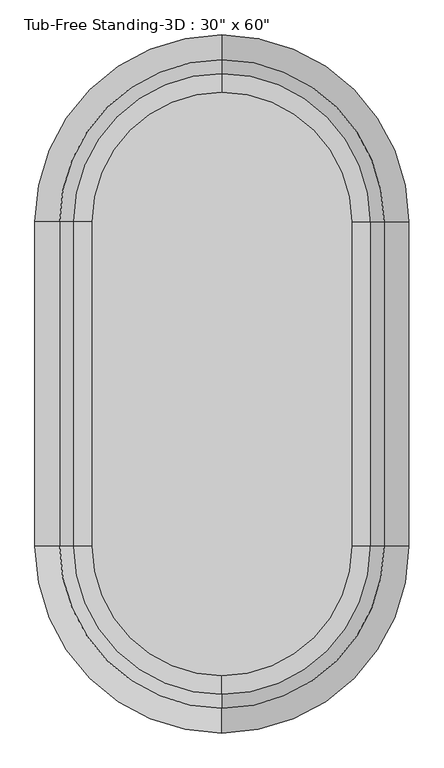
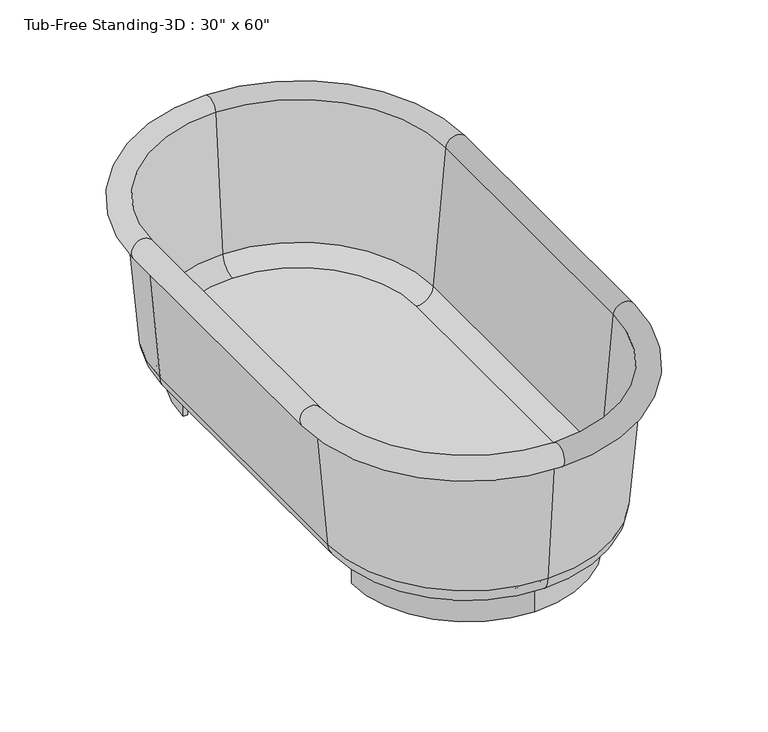
"""IFC4 building model written with IfcOpenShell, lengths in millimetres: flow terminal geometry."""

from ifc_helpers import new_model, si_unit, point, frame, frame_2d, origin, origin_with_axes, place, context, project, spatial, polyline, circle_curve, ellipse_curve, trimmed, segment, composite_curve, outline, extrude, source, transform, mapped, element, save
from ifc_brep_helpers import plane_surface, cylinder_surface, revolved_surface, advanced_brep


def flow_terminal_a2f06f5b(model_context):
    return source(origin(), model_context, "Body", "SolidModel", [
        extrude(outline(composite_curve([segment(trimmed(circle_curve(frame_2d((0.0, 330.2)), 254.0), [point((0.0, 584.2))], [point((-254.0, 330.2))], True, "CARTESIAN"), True, "CONTINUOUS"), segment(polyline([(-254.0, 330.2), (-264.2824236, 330.2)]), True, "CONTINUOUS"), segment(trimmed(circle_curve(frame_2d((0.0, 330.2)), 264.2824236), [point((-264.2824236, 330.2))], [point((0.0, 594.4824236))], False, "CARTESIAN"), True, "CONTINUOUS"), segment(trimmed(circle_curve(frame_2d((0.0, 330.2)), 264.2824236), [point((0.0, 594.4824236))], [point((264.2824236, 330.2))], False, "CARTESIAN"), True, "CONTINUOUS"), segment(polyline([(264.2824236, 330.2), (254.0, 330.2)]), True, "CONTINUOUS"), segment(trimmed(circle_curve(frame_2d((0.0, 330.2)), 254.0), [point((254.0, 330.2))], [point((0.0, 584.2))], True, "CARTESIAN"), True, "CONTINUOUS")], self_intersect=False)), origin_with_axes(), (0.0, 0.0, 1.0), 63.5),
        extrude(outline(composite_curve([segment(trimmed(circle_curve(frame_2d((0.0, -330.2)), 264.2824236), [point((0.0, -594.4824236))], [point((-264.2824236, -330.2))], False, "CARTESIAN"), True, "CONTINUOUS"), segment(polyline([(-264.2824236, -330.2), (-254.0, -330.2)]), True, "CONTINUOUS"), segment(trimmed(circle_curve(frame_2d((0.0, -330.2)), 254.0), [point((-254.0, -330.2))], [point((0.0, -584.2))], True, "CARTESIAN"), True, "CONTINUOUS"), segment(trimmed(circle_curve(frame_2d((0.0, -330.2)), 254.0), [point((0.0, -584.2))], [point((254.0, -330.2))], True, "CARTESIAN"), True, "CONTINUOUS"), segment(polyline([(254.0, -330.2), (264.2824236, -330.2)]), True, "CONTINUOUS"), segment(trimmed(circle_curve(frame_2d((0.0, -330.2)), 264.2824236), [point((264.2824236, -330.2))], [point((0.0, -594.4824236))], False, "CARTESIAN"), True, "CONTINUOUS")], self_intersect=False)), origin_with_axes(), (0.0, 0.0, 1.0), 63.5),
        extrude(outline(composite_curve([segment(polyline([(-264.2824236, -330.2), (-264.2824236, 330.2)]), True, "CONTINUOUS"), segment(trimmed(circle_curve(frame_2d((0.0, 330.2)), 264.2824236), [point((-264.2824236, 330.2))], [point((0.0, 594.4824236))], False, "CARTESIAN"), True, "CONTINUOUS"), segment(trimmed(circle_curve(frame_2d((0.0, 330.2)), 264.2824236), [point((0.0, 594.4824236))], [point((264.2824236, 330.2))], False, "CARTESIAN"), True, "CONTINUOUS"), segment(polyline([(264.2824236, 330.2), (264.2824236, -330.2)]), True, "CONTINUOUS"), segment(trimmed(circle_curve(frame_2d((0.0, -330.2)), 264.2824236), [point((264.2824236, -330.2))], [point((0.0, -594.4824236))], False, "CARTESIAN"), True, "CONTINUOUS"), segment(trimmed(circle_curve(frame_2d((0.0, -330.2)), 264.2824236), [point((0.0, -594.4824236))], [point((-264.2824236, -330.2))], False, "CARTESIAN"), True, "CONTINUOUS")], self_intersect=False)), frame((0.0, 0.0, 63.5), z_axis=(0.0, 0.0, 1.0), x_axis=(1.0, 0.0, 0.0)), (0.0, 0.0, 1.0), 15.08125),
        advanced_brep(
        [(0.0, -673.1, 406.4), (342.9, -330.2, 406.4), (355.6, -330.2, 406.4), (0.0, -685.8, 406.4), (0.0, -647.3045038, 111.5561295), (317.1045038, -330.2, 111.5561295), (0.0, -594.4824236, 63.1536107), (264.2824236, -330.2, 63.1536107), (0.0, -594.4824236, 78.0774627), (264.2824236, -330.2, 78.0774627), (0.0, -632.4374416, 112.8568289), (302.2374416, -330.2, 112.8568289), (0.0, -660.6561556, 435.3982063), (330.4561556, -330.2, 435.3982063), (-342.9, -330.2, 406.4), (-355.6, -330.2, 406.4), (-317.1045038, -330.2, 111.5561295), (-264.2824236, -330.2, 63.1536107), (-264.2824236, -330.2, 78.0774627), (-302.2374416, -330.2, 112.8568289), (-330.4561556, -330.2, 435.3982063), (-355.6, 330.2, 406.4), (-342.9, 330.2, 406.4), (-317.1045038, 330.2, 111.5561295), (-264.2824236, 330.2, 63.1536107), (-264.2824236, 330.2, 78.0774627), (-302.2374416, 330.2, 112.8568289), (-330.4561556, 330.2, 435.3982063), (0.0, 673.1, 406.4), (0.0, 685.8, 406.4), (0.0, 647.3045038, 111.5561295), (0.0, 594.4824236, 63.1536107), (0.0, 594.4824236, 78.0774627), (0.0, 632.4374416, 112.8568289), (0.0, 660.6561556, 435.3982063), (342.9, 330.2, 406.4), (355.6, 330.2, 406.4), (317.1045038, 330.2, 111.5561295), (264.2824236, 330.2, 63.1536107), (264.2824236, 330.2, 78.0774627), (302.2374416, 330.2, 112.8568289), (330.4561556, 330.2, 435.3982063)],
        [
            (0, 1, circle_curve(frame((0.0, -330.2, 406.4), z_axis=(0.0, 0.0, 1.0), x_axis=(1.0, 0.0, 0.0)), 342.9)),
            (1, 2),
            (2, 3, circle_curve(frame((0.0, -330.2, 406.4), z_axis=(0.0, 0.0, -1.0), x_axis=(1.0, 0.0, 0.0)), 355.6)),
            (3, 0),
            (4, 5, circle_curve(frame((0.0, -330.2, 111.5561295), z_axis=(0.0, 0.0, 1.0), x_axis=(1.0, 0.0, 0.0)), 317.1045038)),
            (5, 1),
            (0, 4),
            (6, 7, circle_curve(frame((0.0, -330.2, 63.1536107), z_axis=(0.0, 0.0, 1.0), x_axis=(1.0, 0.0, 0.0)), 264.2824236)),
            (7, 5, circle_curve(frame((264.2824236, -330.2, 116.1774627), z_axis=(0.0, -1.0, 0.0), x_axis=(1.0, 0.0, 0.0)), 53.023852)),
            (4, 6, circle_curve(frame((0.0, -594.4824236, 116.1774627), z_axis=(1.0, 0.0, 0.0), x_axis=(0.0, -1.0, 0.0)), 53.023852)),
            (8, 9, circle_curve(frame((0.0, -330.2, 78.0774627), z_axis=(0.0, 0.0, 1.0), x_axis=(1.0, 0.0, 0.0)), 264.2824236)),
            (9, 7),
            (6, 8),
            (10, 11, circle_curve(frame((0.0, -330.2, 112.8568289), z_axis=(0.0, 0.0, 1.0), x_axis=(1.0, 0.0, 0.0)), 302.2374416)),
            (11, 9, circle_curve(frame((264.2824236, -330.2, 116.1774627), z_axis=(0.0, 1.0, 0.0), x_axis=(1.0, 0.0, 0.0)), 38.1)),
            (8, 10, circle_curve(frame((0.0, -594.4824236, 116.1774627), z_axis=(-1.0, 0.0, 0.0), x_axis=(0.0, -1.0, 0.0)), 38.1)),
            (12, 13, circle_curve(frame((0.0, -330.2, 435.3982063), z_axis=(0.0, 0.0, 1.0), x_axis=(1.0, 0.0, 0.0)), 330.4561556)),
            (13, 11),
            (10, 12),
            (2, 13, circle_curve(frame((355.6, -330.2, 431.8), z_axis=(0.0, -1.0, 0.0), x_axis=(1.0, 0.0, 0.0)), 25.4)),
            (12, 3, circle_curve(frame((0.0, -685.8, 431.8), z_axis=(1.0, 0.0, 0.0), x_axis=(0.0, -1.0, 0.0)), 25.4)),
            (14, 0, circle_curve(frame((0.0, -330.2, 406.4), z_axis=(0.0, 0.0, 1.0), x_axis=(0.0, -1.0, 0.0)), 342.9)),
            (3, 15, circle_curve(frame((0.0, -330.2, 406.4), z_axis=(0.0, 0.0, -1.0), x_axis=(0.0, -1.0, 0.0)), 355.6)),
            (15, 14),
            (16, 4, circle_curve(frame((0.0, -330.2, 111.5561295), z_axis=(0.0, 0.0, 1.0), x_axis=(0.0, -1.0, 0.0)), 317.1045038)),
            (14, 16),
            (17, 6, circle_curve(frame((0.0, -330.2, 63.1536107), z_axis=(0.0, 0.0, 1.0), x_axis=(0.0, -1.0, 0.0)), 264.2824236)),
            (16, 17, circle_curve(frame((-264.2824236, -330.2, 116.1774627), z_axis=(0.0, -1.0, 0.0), x_axis=(-1.0, 0.0, 0.0)), 53.023852)),
            (18, 8, circle_curve(frame((0.0, -330.2, 78.0774627), z_axis=(0.0, 0.0, 1.0), x_axis=(0.0, -1.0, 0.0)), 264.2824236)),
            (17, 18),
            (19, 10, circle_curve(frame((0.0, -330.2, 112.8568289), z_axis=(0.0, 0.0, 1.0), x_axis=(0.0, -1.0, 0.0)), 302.2374416)),
            (18, 19, circle_curve(frame((-264.2824236, -330.2, 116.1774627), z_axis=(0.0, 1.0, 0.0), x_axis=(-1.0, 0.0, 0.0)), 38.1)),
            (20, 12, circle_curve(frame((0.0, -330.2, 435.3982063), z_axis=(0.0, 0.0, 1.0), x_axis=(0.0, -1.0, 0.0)), 330.4561556)),
            (19, 20),
            (20, 15, circle_curve(frame((-355.6, -330.2, 431.8), z_axis=(0.0, -1.0, 0.0), x_axis=(-1.0, 0.0, 0.0)), 25.4)),
            (15, 21),
            (21, 22),
            (22, 14),
            (22, 23),
            (23, 16),
            (23, 24, circle_curve(frame((-264.2824236, 330.2, 116.1774627), z_axis=(0.0, -1.0, 0.0), x_axis=(-1.0, 0.0, 0.0)), 53.023852)),
            (24, 17),
            (24, 25),
            (25, 18),
            (25, 26, circle_curve(frame((-264.2824236, 330.2, 116.1774627), z_axis=(0.0, 1.0, 0.0), x_axis=(-1.0, 0.0, 0.0)), 38.1)),
            (26, 19),
            (26, 27),
            (27, 20),
            (27, 21, circle_curve(frame((-355.6, 330.2, 431.8), z_axis=(0.0, -1.0, 0.0), x_axis=(-1.0, 0.0, 0.0)), 25.4)),
            (28, 22, circle_curve(frame((0.0, 330.2, 406.4), z_axis=(0.0, 0.0, 1.0), x_axis=(-1.0, 0.0, 0.0)), 342.9)),
            (21, 29, circle_curve(frame((0.0, 330.2, 406.4), z_axis=(0.0, 0.0, -1.0), x_axis=(-1.0, 0.0, 0.0)), 355.6)),
            (29, 28),
            (30, 23, circle_curve(frame((0.0, 330.2, 111.5561295), z_axis=(0.0, 0.0, 1.0), x_axis=(-1.0, 0.0, 0.0)), 317.1045038)),
            (28, 30),
            (31, 24, circle_curve(frame((0.0, 330.2, 63.1536107), z_axis=(0.0, 0.0, 1.0), x_axis=(-1.0, 0.0, 0.0)), 264.2824236)),
            (30, 31, circle_curve(frame((0.0, 594.4824236, 116.1774627), z_axis=(-1.0, 0.0, 0.0), x_axis=(0.0, 1.0, 0.0)), 53.023852)),
            (32, 25, circle_curve(frame((0.0, 330.2, 78.0774627), z_axis=(0.0, 0.0, 1.0), x_axis=(-1.0, 0.0, 0.0)), 264.2824236)),
            (31, 32),
            (33, 26, circle_curve(frame((0.0, 330.2, 112.8568289), z_axis=(0.0, 0.0, 1.0), x_axis=(-1.0, 0.0, 0.0)), 302.2374416)),
            (32, 33, circle_curve(frame((0.0, 594.4824236, 116.1774627), z_axis=(1.0, 0.0, 0.0), x_axis=(0.0, 1.0, 0.0)), 38.1)),
            (34, 27, circle_curve(frame((0.0, 330.2, 435.3982063), z_axis=(0.0, 0.0, 1.0), x_axis=(-1.0, 0.0, 0.0)), 330.4561556)),
            (33, 34),
            (34, 29, circle_curve(frame((0.0, 685.8, 431.8), z_axis=(-1.0, 0.0, 0.0), x_axis=(0.0, 1.0, 0.0)), 25.4)),
            (35, 28, circle_curve(frame((0.0, 330.2, 406.4), z_axis=(0.0, 0.0, 1.0), x_axis=(0.0, 1.0, 0.0)), 342.9)),
            (29, 36, circle_curve(frame((0.0, 330.2, 406.4), z_axis=(0.0, 0.0, -1.0), x_axis=(0.0, 1.0, 0.0)), 355.6)),
            (36, 35),
            (37, 30, circle_curve(frame((0.0, 330.2, 111.5561295), z_axis=(0.0, 0.0, 1.0), x_axis=(0.0, 1.0, 0.0)), 317.1045038)),
            (35, 37),
            (38, 31, circle_curve(frame((0.0, 330.2, 63.1536107), z_axis=(0.0, 0.0, 1.0), x_axis=(0.0, 1.0, 0.0)), 264.2824236)),
            (37, 38, circle_curve(frame((264.2824236, 330.2, 116.1774627), z_axis=(0.0, 1.0, 0.0), x_axis=(1.0, 0.0, 0.0)), 53.023852)),
            (39, 32, circle_curve(frame((0.0, 330.2, 78.0774627), z_axis=(0.0, 0.0, 1.0), x_axis=(0.0, 1.0, 0.0)), 264.2824236)),
            (38, 39),
            (40, 33, circle_curve(frame((0.0, 330.2, 112.8568289), z_axis=(0.0, 0.0, 1.0), x_axis=(0.0, 1.0, 0.0)), 302.2374416)),
            (39, 40, circle_curve(frame((264.2824236, 330.2, 116.1774627), z_axis=(0.0, -1.0, 0.0), x_axis=(1.0, 0.0, 0.0)), 38.1)),
            (41, 34, circle_curve(frame((0.0, 330.2, 435.3982063), z_axis=(0.0, 0.0, 1.0), x_axis=(0.0, 1.0, 0.0)), 330.4561556)),
            (40, 41),
            (41, 36, circle_curve(frame((355.6, 330.2, 431.8), z_axis=(0.0, 1.0, 0.0), x_axis=(1.0, 0.0, 0.0)), 25.4)),
            (36, 2),
            (1, 35),
            (5, 37),
            (7, 38),
            (9, 39),
            (11, 40),
            (13, 41),
        ],
        [
            plane_surface(frame((0.0, -330.2, 406.4), z_axis=(0.0, 0.0, -1.0), x_axis=(1.0, 0.0, 0.0))),
            revolved_surface(polyline([(342.9, -330.2, 406.4), (317.1045038, -330.2, 111.5561295)]), (0.0, -330.2, 431.8), (0.0, 0.0, -1.0)),
            revolved_surface(trimmed(ellipse_curve(frame((264.2824236, -330.2, 116.1774627), z_axis=(0.0, 1.0, 0.0), x_axis=(1.0, 0.0, 0.0)), 53.023852, 53.023852), [point((317.1045038, -330.2, 111.5561295))], [point((264.2824236, -330.2, 63.1536107))], True, "CARTESIAN"), (0.0, -330.2, 431.8), (0.0, 0.0, -1.0)),
            revolved_surface(polyline([(264.2824236, -330.2, 63.1536107), (264.2824236, -330.2, 78.07746270000001)]), (0.0, -330.2, 431.8), (0.0, 0.0, -1.0)),
            revolved_surface(trimmed(ellipse_curve(frame((264.2824236, -330.2, 116.1774627), z_axis=(0.0, -1.0, 0.0), x_axis=(1.0, 0.0, 0.0)), 38.1, 38.1), [point((264.2824236, -330.2, 78.0774627))], [point((302.2374416, -330.2, 112.8568289))], True, "CARTESIAN"), (0.0, -330.2, 431.8), (0.0, 0.0, -1.0)),
            revolved_surface(polyline([(302.2374416, -330.2, 112.8568289), (330.4561556, -330.2, 435.3982063)]), (0.0, -330.2, 431.8), (0.0, 0.0, -1.0)),
            revolved_surface(trimmed(ellipse_curve(frame((355.6, -330.2, 431.8), z_axis=(0.0, 1.0, 0.0), x_axis=(1.0, 0.0, 0.0)), 25.4, 25.4), [point((330.4561556, -330.2, 435.3982063))], [point((355.6, -330.2, 406.4))], True, "CARTESIAN"), (0.0, -330.2, 431.8), (0.0, 0.0, -1.0)),
            plane_surface(frame((0.0, -330.2, 406.4), z_axis=(0.0, 0.0, -1.0), x_axis=(0.0, -1.0, 0.0))),
            revolved_surface(polyline([(0.0, -673.1, 406.4), (0.0, -647.3045038, 111.5561295)]), (0.0, -330.2, 431.8), (0.0, 0.0, -1.0)),
            revolved_surface(trimmed(ellipse_curve(frame((0.0, -594.4824236, 116.1774627), z_axis=(1.0, 0.0, 0.0), x_axis=(0.0, -1.0, 0.0)), 53.023852, 53.023852), [point((0.0, -647.3045038, 111.5561295))], [point((0.0, -594.4824236, 63.1536107))], True, "CARTESIAN"), (0.0, -330.2, 431.8), (0.0, 0.0, -1.0)),
            revolved_surface(polyline([(0.0, -594.4824236, 63.1536107), (0.0, -594.4824236, 78.07746270000001)]), (0.0, -330.2, 431.8), (0.0, 0.0, -1.0)),
            revolved_surface(trimmed(ellipse_curve(frame((0.0, -594.4824236, 116.1774627), z_axis=(-1.0, 0.0, 0.0), x_axis=(0.0, -1.0, 0.0)), 38.1, 38.1), [point((0.0, -594.4824236, 78.0774627))], [point((0.0, -632.4374416, 112.8568289))], True, "CARTESIAN"), (0.0, -330.2, 431.8), (0.0, 0.0, -1.0)),
            revolved_surface(polyline([(0.0, -632.4374416, 112.8568289), (0.0, -660.6561556, 435.3982063)]), (0.0, -330.2, 431.8), (0.0, 0.0, -1.0)),
            revolved_surface(trimmed(ellipse_curve(frame((0.0, -685.8, 431.8), z_axis=(1.0, 0.0, 0.0), x_axis=(0.0, -1.0, 0.0)), 25.4, 25.4), [point((0.0, -660.6561556, 435.3982063))], [point((0.0, -685.8, 406.4))], True, "CARTESIAN"), (0.0, -330.2, 431.8), (0.0, 0.0, -1.0)),
            plane_surface(frame((-355.6, -330.2, 406.4), z_axis=(0.0, 0.0, -1.0), x_axis=(0.0, 1.0, 0.0))),
            plane_surface(frame((-342.9, -330.2, 406.4), z_axis=(-0.9961946980917455, 0.0, -0.08715574274765871), x_axis=(0.0, 1.0, 0.0))),
            cylinder_surface(frame((-264.2824236, -330.2, 116.1774627), z_axis=(0.0, -1.0, 0.0), x_axis=(-1.0, 0.0, 0.0)), 53.023852),
            plane_surface(frame((-264.2824236, -330.2, 63.1536107), z_axis=(1.0, 0.0, 0.0), x_axis=(0.0, 1.0, 0.0))),
            revolved_surface(polyline([(-302.38242360000004, 330.2, 116.1774627), (-302.38242360000004, -330.2, 116.1774627)]), (-264.2824236, -330.2, 116.1774627), (0.0, 1.0, 0.0)),
            plane_surface(frame((-302.2374416, -330.2, 112.8568289), z_axis=(0.9961946980917458, 0.0, 0.08715574274765651), x_axis=(0.0, 1.0, 0.0))),
            cylinder_surface(frame((-355.6, -330.2, 431.8), z_axis=(0.0, -1.0, 0.0), x_axis=(-1.0, 0.0, 0.0)), 25.4),
            plane_surface(frame((0.0, 330.2, 406.4), z_axis=(0.0, 0.0, -1.0), x_axis=(-1.0, 0.0, 0.0))),
            revolved_surface(polyline([(-342.9, 330.2, 406.4), (-317.1045038, 330.2, 111.5561295)]), (0.0, 330.2, 431.8), (0.0, 0.0, -1.0)),
            revolved_surface(trimmed(ellipse_curve(frame((-264.2824236, 330.2, 116.1774627), z_axis=(0.0, -1.0, 0.0), x_axis=(-1.0, 0.0, 0.0)), 53.023852, 53.023852), [point((-317.1045038, 330.2, 111.5561295))], [point((-264.2824236, 330.2, 63.1536107))], True, "CARTESIAN"), (0.0, 330.2, 431.8), (0.0, 0.0, -1.0)),
            revolved_surface(polyline([(-264.2824236, 330.2, 63.1536107), (-264.2824236, 330.2, 78.07746270000001)]), (0.0, 330.2, 431.8), (0.0, 0.0, -1.0)),
            revolved_surface(trimmed(ellipse_curve(frame((-264.2824236, 330.2, 116.1774627), z_axis=(0.0, 1.0, 0.0), x_axis=(-1.0, 0.0, 0.0)), 38.1, 38.1), [point((-264.2824236, 330.2, 78.0774627))], [point((-302.2374416, 330.2, 112.8568289))], True, "CARTESIAN"), (0.0, 330.2, 431.8), (0.0, 0.0, -1.0)),
            revolved_surface(polyline([(-302.2374416, 330.2, 112.8568289), (-330.4561556, 330.2, 435.3982063)]), (0.0, 330.2, 431.8), (0.0, 0.0, -1.0)),
            revolved_surface(trimmed(ellipse_curve(frame((-355.6, 330.2, 431.8), z_axis=(0.0, -1.0, 0.0), x_axis=(-1.0, 0.0, 0.0)), 25.4, 25.4), [point((-330.4561556, 330.2, 435.3982063))], [point((-355.6, 330.2, 406.4))], True, "CARTESIAN"), (0.0, 330.2, 431.8), (0.0, 0.0, -1.0)),
            plane_surface(frame((0.0, 330.2, 406.4), z_axis=(0.0, 0.0, -1.0), x_axis=(0.0, 1.0, 0.0))),
            revolved_surface(polyline([(0.0, 673.1, 406.4), (0.0, 647.3045038, 111.5561295)]), (0.0, 330.2, 431.8), (0.0, 0.0, -1.0)),
            revolved_surface(trimmed(ellipse_curve(frame((0.0, 594.4824236, 116.1774627), z_axis=(-1.0, 0.0, 0.0), x_axis=(0.0, 1.0, 0.0)), 53.023852, 53.023852), [point((0.0, 647.3045038, 111.5561295))], [point((0.0, 594.4824236, 63.1536107))], True, "CARTESIAN"), (0.0, 330.2, 431.8), (0.0, 0.0, -1.0)),
            revolved_surface(polyline([(0.0, 594.4824236, 63.1536107), (0.0, 594.4824236, 78.07746270000001)]), (0.0, 330.2, 431.8), (0.0, 0.0, -1.0)),
            revolved_surface(trimmed(ellipse_curve(frame((0.0, 594.4824236, 116.1774627), z_axis=(1.0, 0.0, 0.0), x_axis=(0.0, 1.0, 0.0)), 38.1, 38.1), [point((0.0, 594.4824236, 78.0774627))], [point((0.0, 632.4374416, 112.8568289))], True, "CARTESIAN"), (0.0, 330.2, 431.8), (0.0, 0.0, -1.0)),
            revolved_surface(polyline([(0.0, 632.4374416, 112.8568289), (0.0, 660.6561556, 435.3982063)]), (0.0, 330.2, 431.8), (0.0, 0.0, -1.0)),
            revolved_surface(trimmed(ellipse_curve(frame((0.0, 685.8, 431.8), z_axis=(-1.0, 0.0, 0.0), x_axis=(0.0, 1.0, 0.0)), 25.4, 25.4), [point((0.0, 660.6561556, 435.3982063))], [point((0.0, 685.8, 406.4))], True, "CARTESIAN"), (0.0, 330.2, 431.8), (0.0, 0.0, -1.0)),
            plane_surface(frame((355.6, 330.2, 406.4), z_axis=(0.0, 0.0, -1.0), x_axis=(0.0, -1.0, 0.0))),
            plane_surface(frame((342.9, 330.2, 406.4), z_axis=(0.9961946980917455, 0.0, -0.08715574274765871), x_axis=(0.0, -1.0, 0.0))),
            cylinder_surface(frame((264.2824236, 330.2, 116.1774627), z_axis=(0.0, 1.0, 0.0), x_axis=(1.0, 0.0, 0.0)), 53.023852),
            plane_surface(frame((264.2824236, 330.2, 63.1536107), z_axis=(-1.0, 0.0, 0.0), x_axis=(0.0, -1.0, 0.0))),
            revolved_surface(polyline([(302.38242360000004, -330.2, 116.1774627), (302.38242360000004, 330.2, 116.1774627)]), (264.2824236, 330.2, 116.1774627), (0.0, -1.0, 0.0)),
            plane_surface(frame((302.2374416, 330.2, 112.8568289), z_axis=(-0.9961946980917458, 0.0, 0.08715574274765651), x_axis=(0.0, -1.0, 0.0))),
            cylinder_surface(frame((355.6, 330.2, 431.8), z_axis=(0.0, 1.0, 0.0), x_axis=(1.0, 0.0, 0.0)), 25.4),
        ],
        [
            (0, [[1, 2, 3, 4]]),
            (1, [[5, 6, -1, 7]]),
            (2, [[8, 9, -5, 10]]),
            (3, [[11, 12, -8, 13]]),
            (4, [[14, 15, -11, 16]]),
            (5, [[17, 18, -14, 19]]),
            (6, [[-3, 20, -17, 21]]),
            (7, [[22, -4, 23, 24]]),
            (8, [[25, -7, -22, 26]]),
            (9, [[27, -10, -25, 28]]),
            (10, [[29, -13, -27, 30]]),
            (11, [[31, -16, -29, 32]]),
            (12, [[33, -19, -31, 34]]),
            (13, [[-23, -21, -33, 35]]),
            (14, [[-24, 36, 37, 38]]),
            (15, [[-26, -38, 39, 40]]),
            (16, [[-28, -40, 41, 42]]),
            (17, [[-30, -42, 43, 44]]),
            (18, [[-32, -44, 45, 46]]),
            (19, [[-34, -46, 47, 48]]),
            (20, [[-35, -48, 49, -36]]),
            (21, [[50, -37, 51, 52]]),
            (22, [[53, -39, -50, 54]]),
            (23, [[55, -41, -53, 56]]),
            (24, [[57, -43, -55, 58]]),
            (25, [[59, -45, -57, 60]]),
            (26, [[61, -47, -59, 62]]),
            (27, [[-51, -49, -61, 63]]),
            (28, [[64, -52, 65, 66]]),
            (29, [[67, -54, -64, 68]]),
            (30, [[69, -56, -67, 70]]),
            (31, [[71, -58, -69, 72]]),
            (32, [[73, -60, -71, 74]]),
            (33, [[75, -62, -73, 76]]),
            (34, [[-65, -63, -75, 77]]),
            (35, [[-66, 78, -2, 79]]),
            (36, [[-68, -79, -6, 80]]),
            (37, [[-70, -80, -9, 81]]),
            (38, [[-72, -81, -12, 82]]),
            (39, [[-74, -82, -15, 83]]),
            (40, [[-76, -83, -18, 84]]),
            (41, [[-77, -84, -20, -78]]),
        ],
    ),
    ])


if __name__ == "__main__":
    model = new_model("IFC4")
    model_context = context("Model", 3, world=origin())
    ifc_project = project(units=[si_unit("LENGTHUNIT", "METRE", prefix="MILLI")], contexts=[model_context])
    site = spatial("IfcSite", under=ifc_project)
    building = spatial("IfcBuilding", under=site)
    placement = place(None, origin())
    flow_terminal_shape = flow_terminal_a2f06f5b(model_context)
    element("IfcFlowTerminal", 1, ObjectType="Tub-Free Standing-3D : 30\" x 60\"", at=placement, inside=building, context=model_context, shape_type="MappedRepresentation", body=[
        mapped(flow_terminal_shape, transform((0.0, 0.0, 0.0), x_axis=(1.0, 0.0, 0.0), y_axis=(0.0, 1.0, 0.0), z_axis=(0.0, 0.0, 1.0))),
    ])
    save(model, "model.ifc")

# Revit data of these elements
# Type "Tub-Free Standing-3D : 30\" x 60\""
#   Assembly Code = "D2010110"
#   Height = 1' - 6"
#   Length = 4' - 8"
#   Width = 2' - 6"
#   Tub Material = Porcelain, Ivory
#   Default Elevation = 0
# Element 1 (IfcFlowTerminal, "Tub-Free Standing-3D : 30\" x 60\"")
#   Materials on its faces: "Porcelain, Ivory"
# Materials
#   "Porcelain, Ivory": class "Ceramic", colour RGB 247 247 239, transparency 0, Description = "Porcelain, ivory", Cost = 0
